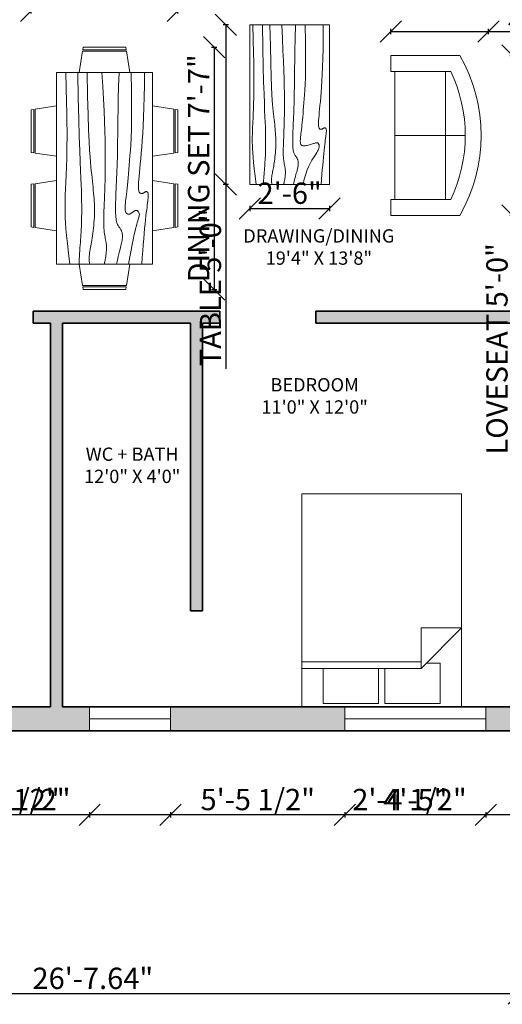
# Model space of a CAD drawing. Units: inches. Extents: x 2561 to 3163, y 493 to 1211.
# Tile 2 of 8: x 2762 to 2943, y 512 to 882. Entities that reach past the tile are written whole.
import ezdxf

# ---------------------------------------------------------------- set-up
doc = ezdxf.new("R2010")
doc.units = ezdxf.units.IN
for name, color, linetype, lineweight in [('A-ANNO-DIMS', 2, 'Continuous', 18), ('A-AREA-IDEN', 7, 'Continuous', 18), ('A-FURN', 8, 'Continuous', 18), ('A-GLAZ', 4, 'Continuous', 18), ('A-WALL', 7, 'Continuous', 35), ('A-WALL-PATT', 24, 'Continuous', 13)]:
    doc.layers.add(name, color=color, linetype=linetype, lineweight=lineweight)
doc.styles.get("Standard").update_dxf_attribs({"font": 'arial.ttf'})
doc.dimstyles.new('ISO-25', dxfattribs={"dimtxt": 8, "dimasz": 8, "dimexe": 1, "dimexo": 1, "dimtad": 1, "dimlunit": 3, "dimtxsty": 'Standard', "dimblk": 'OBLIQUE', "dimcen": 2.5, "dimadec": 0, "dimazin": 0, "dimtfac": 1, "dimtmove": 0, "dimatfit": 3, "dimfxl": 1, "dimfxlon": 1, "dimarcsym": 0})

# ---------------------------------------------------------------- blocks, each defined once
blk = doc.blocks.new('Table - Rectangular Woodgrain 60 x 30 in.')
for p, q in [((0, 0), (0, -30)), ((60, 0), (0, 0)), ((60, -30), (60, 0)), ((0, -30), (60, -30))]:
    blk.add_line(p, q)
for points in [[(0, -2.4), (4.8155, -2.418), (9.0302, -2.4688), (12.709, -2.5477), (15.9167, -2.65), (18.7181, -2.7711), (21.1781, -2.9063), (23.3616, -3.0508), (25.3333, -3.2), (27.1477, -3.3495), (28.8172, -3.4958), (30.3437, -3.636), (31.7291, -3.7667), (32.9756, -3.8849), (34.0849, -3.9875), (35.059, -4.0714), (35.9, -4.1334), (36.6114, -4.1711), (37.2041, -4.1854), (37.6906, -4.1779), (38.0833, -4.15), (38.3948, -4.1034), (38.6375, -4.0396), (38.8239, -3.9602), (38.9666, -3.8667), (39.0764, -3.7608), (39.1573, -3.6448), (39.2116, -3.521), (39.2416, -3.3917), (39.2498, -3.2593), (39.2385, -3.1261), (39.21, -2.9944), (39.1666, -2.8667), (39.111, -2.7447), (39.0468, -2.6281), (38.978, -2.5163), (38.9083, -2.4083), (38.8418, -2.3035), (38.7823, -2.201), (38.7337, -2.1001), (38.7, -2), (38.6844, -1.9003), (38.6875, -1.8021), (38.7094, -1.707), (38.75, -1.6167), (38.8094, -1.5326), (38.8875, -1.4563), (38.9844, -1.3893), (39.1, -1.3333), (39.2351, -1.2896), (39.3937, -1.2583), (39.5804, -1.2396), (39.8, -1.2333), (40.057, -1.2396), (40.3562, -1.2583), (40.7023, -1.2896), (41.1, -1.3333), (41.5547, -1.3895), (42.0755, -1.4573), (42.6721, -1.5361), (43.3542, -1.625), (44.1316, -1.7233), (45.014, -1.8302), (46.0114, -1.9449), (47.1333, -2.0667), (48.3862, -2.1947), (49.7625, -2.3281), (51.2513, -2.4663), (52.8416, -2.6083), (54.5226, -2.7535), (56.2833, -2.9011), (58.1127, -3.0501), (60, -3.2)], [(0, -9.2), (6.5759, -9.0858), (11.9385, -9.0365), (16.2527, -9.0418), (19.6833, -9.0917), (22.3952, -9.1759), (24.5531, -9.2844), (26.322, -9.4069), (27.8666, -9.5333), (29.3241, -9.6553), (30.7203, -9.7719), (32.0532, -9.8837), (33.3208, -9.9917), (34.5213, -10.0965), (35.6526, -10.199), (36.7128, -10.2999), (37.7, -10.4), (38.6129, -10.4996), (39.4531, -10.5969), (40.223, -10.6895), (40.925, -10.775), (41.5613, -10.8512), (42.1344, -10.9156), (42.6465, -10.966), (43.1, -11), (43.4976, -11.0158), (43.8437, -11.0136), (44.143, -10.9942), (44.4, -10.9583), (44.6195, -10.9069), (44.8062, -10.8406), (44.9648, -10.7603), (45.1, -10.6667), (45.2155, -10.5598), (45.3114, -10.4365), (45.3871, -10.2929), (45.4416, -10.125), (45.4743, -9.929), (45.4844, -9.7011), (45.4709, -9.4371), (45.4333, -9.1333), (45.3716, -8.7883), (45.2896, -8.4104), (45.1919, -8.0107), (45.0833, -7.6), (44.9685, -7.1893), (44.8521, -6.7896), (44.7388, -6.4117), (44.6333, -6.0667), (44.54, -5.7628), (44.4614, -5.4979), (44.4001, -5.2675), (44.3583, -5.0667), (44.3384, -4.8909), (44.3427, -4.7354), (44.3736, -4.5956), (44.4333, -4.4667), (44.5236, -4.3453), (44.6427, -4.2333), (44.7884, -4.1339), (44.9583, -4.05), (45.1501, -3.9849), (45.3614, -3.9417), (45.59, -3.9234), (45.8333, -3.9333), (46.0915, -3.9749), (46.3734, -4.0531), (46.6906, -4.1736), (47.0542, -4.3417), (47.4756, -4.5629), (47.9661, -4.8427), (48.5372, -5.1866), (49.2, -5.6), (49.9676, -6.0844), (50.8594, -6.625), (51.8965, -7.2031), (53.1, -7.8), (54.491, -8.3969), (56.0906, -8.975), (57.9199, -9.5156), (60, -10)], [(0, -12.8), (5.1847, -12.9322), (9.6213, -13.0323), (13.3963, -13.1059), (16.5958, -13.1583), (19.3063, -13.1952), (21.614, -13.2219), (23.6054, -13.2439), (25.3666, -13.2667), (26.9728, -13.2947), (28.4531, -13.3281), (29.8256, -13.3663), (31.1083, -13.4083), (32.3191, -13.4535), (33.476, -13.501), (34.597, -13.5501), (35.7, -13.6), (36.7984, -13.6497), (37.8875, -13.6979), (38.9578, -13.743), (40, -13.7833), (41.0047, -13.8174), (41.9625, -13.8438), (42.864, -13.8607), (43.7, -13.8667), (44.4631, -13.8604), (45.1552, -13.8417), (45.7801, -13.8104), (46.3416, -13.7667), (46.8439, -13.7104), (47.2906, -13.6417), (47.6858, -13.5604), (48.0333, -13.4667), (48.3375, -13.3608), (48.6042, -13.2448), (48.8396, -13.121), (49.05, -12.9917), (49.2417, -12.8593), (49.4208, -12.7261), (49.5937, -12.5944), (49.7667, -12.4667), (49.9452, -12.3451), (50.1323, -12.2313), (50.3303, -12.1268), (50.5416, -12.0333), (50.7686, -11.9524), (51.0135, -11.8854), (51.2788, -11.8341), (51.5666, -11.8), (51.8785, -11.7843), (52.2116, -11.7865), (52.562, -11.8059), (52.926, -11.8417), (53.2998, -11.8931), (53.6795, -11.9594), (54.0614, -12.0397), (54.4416, -12.1333), (54.8223, -12.2401), (55.2293, -12.3625), (55.6942, -12.5037), (56.2489, -12.6667), (56.9251, -12.8547), (57.7545, -13.0708), (58.7689, -13.3182), (60, -13.6)], [(0, -18), (5.124, -17.7273), (9.6609, -17.5057), (13.6705, -17.3303), (17.2125, -17.1958), (20.3467, -17.0973), (23.1328, -17.0297), (25.6307, -16.9878), (27.9, -16.9667), (29.9928, -16.9617), (31.9302, -16.9703), (33.7254, -16.9907), (35.3917, -17.0208), (36.9423, -17.0588), (38.3906, -17.1026), (39.7499, -17.1503), (41.0333, -17.2), (42.2519, -17.2496), (43.4073, -17.2969), (44.4986, -17.3395), (45.525, -17.375), (46.4858, -17.4012), (47.3802, -17.4156), (48.2074, -17.416), (48.9667, -17.4), (49.6583, -17.3662), (50.2872, -17.3167), (50.8595, -17.2547), (51.3812, -17.1833), (51.8584, -17.1057), (52.2971, -17.025), (52.7034, -16.9443), (53.0833, -16.8667), (53.443, -16.7951), (53.789, -16.7313), (54.128, -16.6768), (54.4666, -16.6334), (54.8115, -16.6024), (55.1693, -16.5854), (55.5465, -16.5841), (55.95, -16.6), (56.3828, -16.6337), (56.8346, -16.6823), (57.2915, -16.7418), (57.7396, -16.8084), (58.165, -16.878), (58.5539, -16.9469), (58.8924, -17.0111), (59.1666, -17.0667), (59.3679, -17.1107), (59.5078, -17.1438), (59.6032, -17.1675), (59.6708, -17.1833), (59.7275, -17.193), (59.7901, -17.1979), (59.8753, -17.1998), (60, -17.2)], [(0, -22.4), (8.0098, -22.2501), (14.4094, -22.1011), (19.4168, -21.9535), (23.25, -21.8083), (26.1269, -21.6663), (28.2656, -21.5281), (29.884, -21.3947), (31.2, -21.2667), (32.3967, -21.1448), (33.5172, -21.0292), (34.5697, -20.9198), (35.5625, -20.8167), (36.5037, -20.7198), (37.4015, -20.6292), (38.2642, -20.5448), (39.1, -20.4667), (39.9164, -20.3951), (40.7187, -20.3313), (41.5117, -20.2768), (42.3, -20.2333), (43.0883, -20.2024), (43.8812, -20.1854), (44.6836, -20.1841), (45.5, -20.2), (46.3328, -20.234), (47.1747, -20.2844), (48.0163, -20.3488), (48.8479, -20.425), (49.66, -20.5106), (50.4429, -20.6031), (51.1872, -20.7004), (51.8833, -20.8), (52.5246, -20.8999), (53.1166, -20.9995), (53.6681, -21.0983), (54.1875, -21.1958), (54.6834, -21.2919), (55.1646, -21.3859), (55.6394, -21.4777), (56.1167, -21.5667), (56.6028, -21.6515), (57.0961, -21.7266), (57.5929, -21.7852), (58.0896, -21.8208), (58.5823, -21.8268), (59.0674, -21.7964), (59.5412, -21.723), (60, -21.6)], [(0, -25.2), (8.6355, -25.0504), (15.7026, -24.9031), (21.4049, -24.7606), (25.9458, -24.625), (29.529, -24.4988), (32.3578, -24.3844), (34.6359, -24.284), (36.5667, -24.2), (38.3213, -24.1341), (39.9417, -24.0854), (41.437, -24.0523), (42.8167, -24.0333), (44.0901, -24.0268), (45.2667, -24.0313), (46.3557, -24.0451), (47.3667, -24.0667), (48.309, -24.0947), (49.1928, -24.1287), (50.0284, -24.168), (50.826, -24.2125), (51.5959, -24.2617), (52.3483, -24.3151), (53.0935, -24.3725), (53.8417, -24.4334), (54.6009, -24.497), (55.3699, -24.561), (56.1454, -24.6226), (56.9239, -24.6792), (57.7021, -24.7279), (58.4764, -24.7662), (59.2435, -24.7911), (60, -24.8)], [(0, -28.8), (5.6867, -28.6681), (10.45, -28.5698), (14.407, -28.5012), (17.675, -28.4584), (20.3711, -28.4374), (22.6125, -28.4344), (24.5164, -28.4455), (26.2, -28.4667), (27.762, -28.4947), (29.2276, -28.5281), (30.6033, -28.5663), (31.8958, -28.6084), (33.1118, -28.6535), (34.2578, -28.7011), (35.3405, -28.7501), (36.3666, -28.8), (37.3443, -28.8497), (38.288, -28.8974), (39.2137, -28.9412), (40.1375, -28.9792), (41.0753, -29.0093), (42.0432, -29.0297), (43.0572, -29.0384), (44.1333, -29.0333), (45.2936, -29.0114), (46.5843, -28.9641), (48.0579, -28.8816), (49.7666, -28.7542), (51.7629, -28.5721), (54.0989, -28.3255), (56.8272, -28.0048), (60, -27.6)]]:
    blk.add_lwpolyline(points)
blk = doc.blocks.new('Sofa - Roundback Loveseat 5 ft.')
for p, q in [((0, -32.44198), (0, -5.99998)), ((-24, -33.99998), (-24, -11.46958)), ((-23.9998, -13.38178), (23.99986, -13.38178)), ((24.00004, -33.99998), (24.00004, -11.46958)), ((-24, -32.44198), (24.00004, -32.44198))]:
    blk.add_line(p, q)
for points in [[(-24, -33.99998), (-30, -33.99998), (-30, -7.99998)], [(30.00004, -7.99998), (30.00004, -33.99998), (24.00004, -33.99998)]]:
    blk.add_lwpolyline(points)
for centre, radius, start, end in [((0, -60.24998), 60.24998, 60.13715, 119.8628), ((0, -61.38438), 55.38444, 64.32083, 115.6792)]:
    blk.add_arc(centre, radius, start, end)
blk = doc.blocks.new('Dining Set - 36 x 72 in.')
for p, q in [((-22.2343, 26.00059), (-23.4847, 17.99762)), ((-22.2304, 26), (-5.7608, 26)), ((-22, 27.5), (-22.1562, 26.50042)), ((-5.8416, 26.5), (-22.1534, 26.5)), ((-22, 27.5), (-6, 27.5)), ((-5.8437, 26.49966), (-6, 27.5)), ((-4.5152, 17.99762), (-5.7655, 25.99926)), ((5.7657, 26.00059), (4.5153, 17.99762)), ((5.7696, 26), (22.2392, 26)), ((6, 27.5), (5.8438, 26.50042)), ((22.1584, 26.5), (5.8466, 26.5)), ((6, 27.5), (22, 27.5)), ((22.1563, 26.49966), (22, 27.5)), ((23.4848, 17.99762), (22.2345, 25.99926)), ((36, 18), (-36, 18)), ((-36, 18), (-36, -18)), ((36, -18), (36, 18)), ((-45.5, 8), (-44.5004, 8.15617)), ((-45.5, 8), (-45.5, -8)), ((-44.5, -8.15843), (-44.5, 8.15338)), ((-44.0006, 8.23428), (-35.9976, 9.48474)), ((-44, 8.23041), (-44, -8.23915)), ((44.0006, 8.23428), (35.9976, 9.48474)), ((44, 8.23041), (44, -8.23915)), ((44.5, -8.15843), (44.5, 8.15338)), ((45.5, 8), (44.5005, 8.15617)), ((45.5, 8), (45.5, -8)), ((-44.4997, -8.15631), (-45.5, -8)), ((-35.9976, -9.48476), (-43.9993, -8.2345)), ((35.9976, -9.48476), (43.9993, -8.2345)), ((44.4997, -8.15631), (45.5, -8)), ((-36, -18), (36, -18)), ((-22.2343, -26.0006), (-23.4847, -17.99762)), ((-4.5152, -17.99762), (-5.7655, -25.99928)), ((5.7657, -26.0006), (4.5153, -17.99762)), ((23.4848, -17.99762), (22.2345, -25.99928)), ((-22.2304, -26), (-5.7608, -26)), ((-22, -27.5), (-22.1562, -26.50044)), ((-5.8416, -26.5), (-22.1534, -26.5)), ((-22, -27.5), (-6, -27.5)), ((-5.8437, -26.49967), (-6, -27.5)), ((5.7696, -26), (22.2392, -26)), ((6, -27.5), (5.8438, -26.50044)), ((22.1584, -26.5), (5.8466, -26.5)), ((6, -27.5), (22, -27.5)), ((22.1563, -26.49967), (22, -27.5))]:
    blk.add_line(p, q)
for points in [[(-36, 15), (-31.1772, 14.97754), (-26.8079, 14.91406), (-22.8538, 14.81543), (-19.276, 14.6875), (-16.0362, 14.53613), (-13.0957, 14.36718), (-10.4159, 14.18652), (-7.9583, 14), (-5.6904, 13.81315), (-3.6035, 13.63021), (-1.6954, 13.45508), (0.0365, 13.29166), (1.5945, 13.14388), (2.9811, 13.01562), (4.1988, 12.9108), (5.25, 12.83333), (6.1393, 12.78613), (6.8802, 12.76823), (7.4883, 12.77767), (7.9792, 12.8125), (8.3685, 12.87077), (8.6719, 12.95052), (8.9049, 13.0498), (9.0833, 13.16666), (9.2205, 13.29899), (9.3216, 13.44401), (9.3895, 13.59879), (9.4271, 13.76041), (9.4373, 13.92594), (9.4232, 14.09245), (9.3875, 14.257), (9.3333, 14.41666), (9.2638, 14.56917), (9.1836, 14.71484), (9.0975, 14.85465), (9.0104, 14.98958), (8.9272, 15.1206), (8.8529, 15.2487), (8.7922, 15.37483), (8.75, 15.5), (8.7305, 15.62467), (8.7344, 15.74739), (8.7617, 15.86621), (8.8125, 15.97916), (8.8867, 16.08431), (8.9844, 16.17968), (9.1055, 16.26334), (9.25, 16.33333), (9.4189, 16.38802), (9.6172, 16.42708), (9.8506, 16.45052), (10.125, 16.45833), (10.4463, 16.45052), (10.8203, 16.42708), (11.2529, 16.38802), (11.75, 16.33333), (12.3184, 16.26318), (12.9694, 16.17838), (13.7151, 16.07991), (14.5677, 15.96875), (15.5395, 15.84586), (16.6426, 15.71224), (17.8893, 15.56884), (19.2917, 15.41666), (20.859, 15.25667), (22.5879, 15.08984), (24.4721, 14.91715), (26.5052, 14.73958), (28.6809, 14.5581), (30.9929, 14.3737), (33.4347, 14.18733), (36, 14)], [(-36, 10), (-28.9766, 10.14274), (-23.1725, 10.20442), (-18.4241, 10.19775), (-14.5677, 10.13541), (-11.4399, 10.03011), (-8.877, 9.89453), (-6.7154, 9.74137), (-4.7917, 9.58333), (-2.9698, 9.43082), (-1.2246, 9.28515), (0.4415, 9.14534), (2.026, 9.01041), (3.5266, 8.87939), (4.9408, 8.7513), (6.266, 8.62516), (7.5, 8.5), (8.6411, 8.37549), (9.6914, 8.2539), (10.6538, 8.13818), (11.5312, 8.03125), (12.3267, 7.93603), (13.043, 7.85547), (13.6831, 7.79248), (14.25, 7.75), (14.7471, 7.7303), (15.1797, 7.73307), (15.5537, 7.75732), (15.875, 7.80208), (16.1494, 7.86637), (16.3828, 7.94922), (16.5811, 8.04964), (16.75, 8.16666), (16.8944, 8.29915), (17.0143, 8.44531), (17.1089, 8.60319), (17.1771, 8.77083), (17.218, 8.94629), (17.2305, 9.1276), (17.2137, 9.31282), (17.1667, 9.5), (17.0895, 9.6875), (16.987, 9.875), (16.8649, 10.0625), (16.7292, 10.25), (16.5856, 10.4375), (16.4401, 10.625), (16.2985, 10.8125), (16.1667, 11), (16.05, 11.18733), (15.9518, 11.3737), (15.8752, 11.5581), (15.8229, 11.73958), (15.798, 11.91715), (15.8034, 12.08984), (15.842, 12.25667), (15.9167, 12.41666), (16.0295, 12.56836), (16.1784, 12.70833), (16.3605, 12.83268), (16.5729, 12.9375), (16.8127, 13.01888), (17.0768, 13.07291), (17.3625, 13.0957), (17.6667, 13.08333), (17.9894, 13.03312), (18.3418, 12.94726), (18.7382, 12.82918), (19.1927, 12.68229), (19.7195, 12.51001), (20.3327, 12.31575), (21.0465, 12.10294), (21.875, 11.875), (22.8357, 11.63354), (23.959, 11.37304), (25.2786, 11.08618), (26.8282, 10.76562), (28.6414, 10.40405), (30.752, 9.99414), (33.1936, 9.52856), (36, 9)], [(-36, 5.5), (-30.7157, 5.3348), (-26.069, 5.20963), (-21.9946, 5.11767), (-18.4271, 5.05208), (-15.3009, 5.00602), (-12.5508, 4.97265), (-10.1112, 4.94515), (-7.9167, 4.91666), (-5.909, 4.88167), (-4.0586, 4.83984), (-2.3429, 4.79215), (-0.7396, 4.73958), (0.7739, 4.6831), (2.22, 4.6237), (3.6213, 4.56233), (5, 4.5), (6.373, 4.43782), (7.7344, 4.3776), (9.0723, 4.32129), (10.375, 4.27083), (11.6309, 4.22819), (12.8281, 4.19531), (13.9551, 4.17415), (15, 4.16666), (15.954, 4.17448), (16.819, 4.19791), (17.6001, 4.23698), (18.3021, 4.29166), (18.9299, 4.36198), (19.4883, 4.44791), (19.9823, 4.54948), (20.4167, 4.66666), (20.7969, 4.79899), (21.1302, 4.94401), (21.4245, 5.09879), (21.6875, 5.26041), (21.9271, 5.42594), (22.1511, 5.59245), (22.3672, 5.757), (22.5834, 5.91666), (22.8065, 6.06868), (23.0404, 6.21093), (23.2879, 6.34147), (23.5521, 6.45833), (23.8358, 6.55957), (24.142, 6.64323), (24.4735, 6.70735), (24.8334, 6.75), (25.2235, 6.76969), (25.642, 6.76692), (26.0858, 6.74267), (26.5521, 6.69791), (27.0379, 6.63362), (27.5404, 6.55078), (28.0565, 6.45036), (28.5834, 6.33333), (29.1242, 6.19987), (29.7071, 6.04687), (30.3661, 5.87044), (31.1354, 5.66666), (32.0493, 5.43164), (33.142, 5.16146), (34.4475, 4.85221), (36, 4.5)], [(-36, -1), (-30.7915, -0.6591), (-26.0195, -0.38216), (-21.6519, -0.16284), (-17.6563, 0.00521), (-14.0005, 0.12833), (-10.6523, 0.21289), (-7.5796, 0.26522), (-4.75, 0.29166), (-2.134, 0.29793), (0.2878, 0.28711), (2.5317, 0.26163), (4.6146, 0.22396), (6.5529, 0.17651), (8.3633, 0.12174), (10.0623, 0.06209), (11.6667, 0), (13.1899, -0.06201), (14.6341, -0.1211), (15.9982, -0.17432), (17.2813, -0.21875), (18.4823, -0.25147), (19.6003, -0.26953), (20.6343, -0.27002), (21.5834, -0.25), (22.4481, -0.20768), (23.2357, -0.14584), (23.9549, -0.06836), (24.6146, 0.02083), (25.2235, 0.11784), (25.7904, 0.21875), (26.3241, 0.31966), (26.8334, 0.41666), (27.3265, 0.50618), (27.8099, 0.58593), (28.2894, 0.65397), (28.7709, 0.70833), (29.2601, 0.74707), (29.763, 0.76823), (30.2855, 0.76985), (30.8334, 0.75), (31.4088, 0.70784), (31.9994, 0.64713), (32.589, 0.57275), (33.1615, 0.48958), (33.7008, 0.4025), (34.1908, 0.3164), (34.6153, 0.23616), (34.9584, 0.16666), (35.2099, 0.11165), (35.3848, 0.07031), (35.504, 0.04069), (35.5886, 0.02083), (35.6594, 0.00879), (35.7377, 0.0026), (35.8442, 0.00032), (36, 0)], [(-36, -6.5), (-27.1843, -6.31267), (-20.084, -6.1263), (-14.469, -5.9419), (-10.1094, -5.76042), (-6.7752, -5.58285), (-4.2363, -5.41016), (-2.2629, -5.24333), (-0.625, -5.08334), (0.8708, -4.93099), (2.2715, -4.78646), (3.5872, -4.64974), (4.8281, -4.52084), (6.0046, -4.39974), (7.127, -4.28646), (8.2053, -4.18099), (9.25, -4.08334), (10.2705, -3.99382), (11.2734, -3.91407), (12.2647, -3.84603), (13.25, -3.79167), (14.2354, -3.75293), (15.2266, -3.73177), (16.2295, -3.73015), (17.25, -3.75), (18.2912, -3.79248), (19.3451, -3.85547), (20.4009, -3.93604), (21.4479, -4.03125), (22.4754, -4.13819), (23.4727, -4.25391), (24.4289, -4.37549), (25.3334, -4.5), (26.1785, -4.62492), (26.9694, -4.74935), (27.7145, -4.87281), (28.4219, -4.99479), (29.1, -5.11483), (29.7572, -5.23242), (30.4016, -5.34709), (31.0417, -5.45834), (31.6837, -5.56437), (32.3262, -5.65821), (32.9658, -5.73153), (33.599, -5.77604), (34.2224, -5.78345), (34.8327, -5.74545), (35.4264, -5.65373), (36, -5.5)], [(-36, -10), (-26.4022, -9.81299), (-18.4675, -9.62891), (-11.9839, -9.45069), (-6.7396, -9.28125), (-2.5226, -9.12354), (0.8789, -8.98047), (3.6769, -8.85498), (6.0833, -8.75), (8.2767, -8.66765), (10.3021, -8.60677), (12.1712, -8.56543), (13.8958, -8.54167), (15.4876, -8.53353), (16.9583, -8.53907), (18.3197, -8.55632), (19.5834, -8.58334), (20.7616, -8.61841), (21.8685, -8.66081), (22.9188, -8.71004), (23.9271, -8.76563), (24.9081, -8.82707), (25.8763, -8.89388), (26.8465, -8.96558), (27.8334, -9.04167), (28.8474, -9.12118), (29.8828, -9.20117), (30.93, -9.27824), (31.9792, -9.34896), (33.0205, -9.40991), (34.0443, -9.45768), (35.0407, -9.48885), (36, -9.5)], [(-36, -14.5), (-30.0881, -14.33513), (-25.0332, -14.21224), (-20.7312, -14.12647), (-17.0781, -14.07292), (-13.97, -14.04671), (-11.3027, -14.04297), (-8.9724, -14.05681), (-6.875, -14.08334), (-4.9224, -14.11833), (-3.0905, -14.16016), (-1.3709, -14.20785), (0.2448, -14.26042), (1.7647, -14.3169), (3.1973, -14.3763), (4.5507, -14.43767), (5.8333, -14.5), (7.0554, -14.5621), (8.235, -14.62175), (9.3922, -14.67652), (10.5469, -14.72396), (11.7192, -14.76164), (12.929, -14.78711), (14.1965, -14.79794), (15.5417, -14.79167), (16.9933, -14.76424), (18.6152, -14.70508), (20.4804, -14.60197), (22.6615, -14.44271), (25.2312, -14.21509), (28.2624, -13.9069), (31.8277, -13.50594), (36, -13)]]:
    blk.add_lwpolyline(points)
blk = doc.blocks.new('Bed - Queen')
for p, q in [((0, -80.00003), (0, 0)), ((0, 0), (59.99999, 0)), ((59.99999, 0), (59.99999, -80.00003)), ((7.99999, -1.2), (28.79998, -1.2)), ((7.99999, -14.4), (7.99999, -1.2)), ((28.79998, -1.2), (28.79998, -14.4)), ((31.19999, -1.2), (51.99999, -1.2)), ((31.19999, -14.4), (31.19999, -1.2)), ((51.99999, -1.2), (51.99999, -16.4)), ((0, -14.4), (44.8, -14.4)), ((59.99999, -29.6), (44.8, -14.4)), ((44.8, -14.4), (44.8, -29.6)), ((44.8, -16.8), (0, -16.8)), ((51.99999, -16.4), (46.79936, -16.4)), ((44.8, -29.6), (59.99999, -29.6)), ((59.99999, -80.00003), (0, -80.00003))]:
    blk.add_line(p, q)
blk = doc.blocks.new('_Oblique')
at = {"color": 0, "linetype": 'ByBlock', "lineweight": -2}
blk.add_line((-0.5, -0.5), (0.5, 0.5), dxfattribs=at)
blk = doc.blocks.new('*D15')
at = {"layer": 'A-ANNO-DIMS', "color": 0, "lineweight": -2, "transparency": 16777216}
for p, q in [((2629.27, 516.82), (2629.27, 514.82)), ((2629.27, 515.82), (2948.92, 515.82)), ((2948.92, 516.82), (2948.92, 514.82))]:
    blk.add_line(p, q, dxfattribs=at)
at = {"layer": 'Defpoints', "color": 0, "transparency": 16777216}
for p in [(2629.27, 614.57), (2948.92, 614.57), (2948.92, 515.82)]:
    blk.add_point(p, dxfattribs=at)
at = {"layer": 'A-ANNO-DIMS', "color": 0, "lineweight": -2, "transparency": 16777216, "xscale": 8, "yscale": 8, "zscale": 8, "rotation": 180}
blk.add_blockref('_Oblique', (2629.27, 515.82), dxfattribs=at)
at = {"layer": 'A-ANNO-DIMS', "color": 0, "lineweight": -2, "transparency": 16777216, "xscale": 8, "yscale": 8, "zscale": 8}
blk.add_blockref('_Oblique', (2948.92, 515.82), dxfattribs=at)
at = {"layer": 'A-ANNO-DIMS', "color": 0, "transparency": 16777216, "insert": (2789.1, 520.53), "char_height": 8, "attachment_point": 5}
blk.add_mtext('26\'-7.64"', dxfattribs=at)
blk = doc.blocks.new('*D17')
at = {"layer": 'A-ANNO-DIMS', "color": 0, "lineweight": -2, "transparency": 16777216}
for p, q in [((2571.63, 1093.07), (2569.63, 1093.07)), ((2570.63, 1093.07), (2570.63, 529.07)), ((2571.63, 529.07), (2569.63, 529.07))]:
    blk.add_line(p, q, dxfattribs=at)
at = {"layer": 'Defpoints', "color": 0, "transparency": 16777216}
for p in [(2629.27, 1093.07), (2570.63, 529.07), (3109.27, 529.07)]:
    blk.add_point(p, dxfattribs=at)
at = {"layer": 'A-ANNO-DIMS', "color": 0, "lineweight": -2, "transparency": 16777216, "xscale": 8, "yscale": 8, "zscale": 8}
for p, rotation in [((2570.63, 1093.07), 90), ((2570.63, 529.07), 270)]:
    blk.add_blockref('_Oblique', p, dxfattribs=dict(at, rotation=rotation))
at = {"layer": 'A-ANNO-DIMS', "color": 0, "transparency": 16777216, "insert": (2566, 811.07), "char_height": 8, "attachment_point": 5, "rotation": 90}
blk.add_mtext("47'", dxfattribs=at)
blk = doc.blocks.new('*D24')
at = {"layer": 'A-ANNO-DIMS', "color": 0, "lineweight": -2, "transparency": 16777216}
for p, q in [((2839.96, 879.66), (2837.96, 879.66)), ((2838.96, 879.66), (2838.96, 819.66)), ((2839.96, 819.66), (2837.96, 819.66)), ((2838.96, 819.66), (2838.96, 750.44))]:
    blk.add_line(p, q, dxfattribs=at)
at = {"layer": 'Defpoints', "color": 0, "transparency": 16777216}
for p in [(2847.96, 879.66), (2838.96, 819.66), (2847.96, 819.66)]:
    blk.add_point(p, dxfattribs=at)
at = {"layer": 'A-ANNO-DIMS', "color": 0, "lineweight": -2, "transparency": 16777216, "xscale": 8, "yscale": 8, "zscale": 8}
for p, rotation in [((2838.96, 879.66), 90), ((2838.96, 819.66), 270)]:
    blk.add_blockref('_Oblique', p, dxfattribs=dict(at, rotation=rotation))
at = {"layer": 'A-ANNO-DIMS', "color": 0, "transparency": 16777216, "insert": (2834.25, 781.05), "char_height": 8, "attachment_point": 5, "rotation": 90}
blk.add_mtext('TABLE 5\'-0"', dxfattribs=at)
blk = doc.blocks.new('*D25')
at = {"layer": 'A-ANNO-DIMS', "color": 0, "lineweight": -2, "transparency": 16777216}
for p, q in [((2847.96, 811.66), (2847.96, 809.66)), ((2847.96, 810.66), (2877.96, 810.66)), ((2877.96, 811.66), (2877.96, 809.66))]:
    blk.add_line(p, q, dxfattribs=at)
at = {"layer": 'Defpoints', "color": 0, "transparency": 16777216}
for p in [(2847.96, 819.66), (2877.96, 819.66), (2877.96, 810.66)]:
    blk.add_point(p, dxfattribs=at)
at = {"layer": 'A-ANNO-DIMS', "color": 0, "lineweight": -2, "transparency": 16777216, "xscale": 8, "yscale": 8, "zscale": 8, "rotation": 180}
blk.add_blockref('_Oblique', (2847.96, 810.66), dxfattribs=at)
at = {"layer": 'A-ANNO-DIMS', "color": 0, "lineweight": -2, "transparency": 16777216, "xscale": 8, "yscale": 8, "zscale": 8}
blk.add_blockref('_Oblique', (2877.96, 810.66), dxfattribs=at)
at = {"layer": 'A-ANNO-DIMS', "color": 0, "transparency": 16777216, "insert": (2862.96, 815.37), "char_height": 8, "attachment_point": 5}
blk.add_mtext('2\'-6"', dxfattribs=at)
blk = doc.blocks.new('*D26')
at = {"layer": 'A-ANNO-DIMS', "color": 0, "lineweight": -2, "transparency": 16777216}
for p, q in [((2945.53, 868.1), (2947.53, 868.1)), ((2946.53, 868.1), (2946.53, 808.1)), ((2945.53, 808.1), (2947.53, 808.1)), ((2946.53, 808.1), (2946.53, 715.83))]:
    blk.add_line(p, q, dxfattribs=at)
at = {"layer": 'Defpoints', "color": 0, "transparency": 16777216}
for p in [(2937.53, 868.1), (2937.53, 808.1), (2946.53, 808.1)]:
    blk.add_point(p, dxfattribs=at)
at = {"layer": 'A-ANNO-DIMS', "color": 0, "lineweight": -2, "transparency": 16777216, "xscale": 8, "yscale": 8, "zscale": 8}
for p, rotation in [((2946.53, 868.1), 90), ((2946.53, 808.1), 270)]:
    blk.add_blockref('_Oblique', p, dxfattribs=dict(at, rotation=rotation))
at = {"layer": 'A-ANNO-DIMS', "color": 0, "transparency": 16777216, "insert": (2941.77, 757.96), "char_height": 8, "attachment_point": 5, "rotation": 90}
blk.add_mtext('LOVESEAT 5\'-0"', dxfattribs=at)
blk = doc.blocks.new('*D27')
at = {"layer": 'A-ANNO-DIMS', "color": 0, "lineweight": -2, "transparency": 16777216}
for p, q in [((2900.86, 876.1), (2900.86, 878.1)), ((2900.86, 877.1), (2937.53, 877.1)), ((2937.53, 876.1), (2937.53, 878.1)), ((2937.53, 877.1), (2986.68, 877.1))]:
    blk.add_line(p, q, dxfattribs=at)
at = {"layer": 'Defpoints', "color": 0, "transparency": 16777216}
for p in [(2937.53, 877.1), (2900.86, 868.1), (2937.53, 868.1)]:
    blk.add_point(p, dxfattribs=at)
at = {"layer": 'A-ANNO-DIMS', "color": 0, "lineweight": -2, "transparency": 16777216, "xscale": 8, "yscale": 8, "zscale": 8, "rotation": 180}
blk.add_blockref('_Oblique', (2900.86, 877.1), dxfattribs=at)
at = {"layer": 'A-ANNO-DIMS', "color": 0, "lineweight": -2, "transparency": 16777216, "xscale": 8, "yscale": 8, "zscale": 8}
blk.add_blockref('_Oblique', (2937.53, 877.1), dxfattribs=at)
at = {"layer": 'A-ANNO-DIMS', "color": 0, "transparency": 16777216, "insert": (2966.11, 881.86), "char_height": 8, "attachment_point": 5}
blk.add_mtext('3\'-0 1/2"', dxfattribs=at)
blk = doc.blocks.new('*D28')
at = {"layer": 'A-ANNO-DIMS', "color": 0, "lineweight": -2, "transparency": 16777216}
for p, q in [((2833.61, 871.24), (2835.61, 871.24)), ((2834.61, 871.24), (2834.61, 780.24)), ((2833.61, 780.24), (2835.61, 780.24))]:
    blk.add_line(p, q, dxfattribs=at)
at = {"layer": 'Defpoints', "color": 0, "transparency": 16777216}
for p in [(2820.96, 871.24), (2820.96, 780.24), (2834.61, 780.24)]:
    blk.add_point(p, dxfattribs=at)
at = {"layer": 'A-ANNO-DIMS', "color": 0, "lineweight": -2, "transparency": 16777216, "xscale": 8, "yscale": 8, "zscale": 8}
for p, rotation in [((2834.61, 871.24), 90), ((2834.61, 780.24), 270)]:
    blk.add_blockref('_Oblique', p, dxfattribs=dict(at, rotation=rotation))
at = {"layer": 'A-ANNO-DIMS', "color": 0, "transparency": 16777216, "insert": (2829.85, 825.74), "char_height": 8, "attachment_point": 5, "rotation": 90}
blk.add_mtext('DINING SET 7\'-7"', dxfattribs=at)
blk = doc.blocks.new('*D29')
at = {"layer": 'A-ANNO-DIMS', "color": 0, "lineweight": -2, "transparency": 16777216}
for p, q in [((2765.96, 883.89), (2765.96, 885.89)), ((2765.96, 884.89), (2820.96, 884.89)), ((2820.96, 883.89), (2820.96, 885.89))]:
    blk.add_line(p, q, dxfattribs=at)
at = {"layer": 'Defpoints', "color": 0, "transparency": 16777216}
for p in [(2820.96, 884.89), (2765.96, 871.24), (2820.96, 871.24)]:
    blk.add_point(p, dxfattribs=at)
at = {"layer": 'A-ANNO-DIMS', "color": 0, "lineweight": -2, "transparency": 16777216, "xscale": 8, "yscale": 8, "zscale": 8, "rotation": 180}
blk.add_blockref('_Oblique', (2765.96, 884.89), dxfattribs=at)
at = {"layer": 'A-ANNO-DIMS', "color": 0, "lineweight": -2, "transparency": 16777216, "xscale": 8, "yscale": 8, "zscale": 8}
blk.add_blockref('_Oblique', (2820.96, 884.89), dxfattribs=at)
at = {"layer": 'A-ANNO-DIMS', "color": 0, "transparency": 16777216, "insert": (2793.46, 889.52), "char_height": 8, "attachment_point": 5}
blk.add_mtext('4\'-7"', dxfattribs=at)
blk = doc.blocks.new('*D30')
at = {"layer": 'A-ANNO-DIMS', "color": 0, "lineweight": -2, "transparency": 16777216}
for p, q in [((2598.62, 740.07), (2596.62, 740.07)), ((2597.62, 740.07), (2597.62, 701.07)), ((2598.62, 701.07), (2596.62, 701.07))]:
    blk.add_line(p, q, dxfattribs=at)
at = {"layer": 'Defpoints', "color": 0, "transparency": 16777216}
for p in [(3014.77, 740.07), (2597.62, 701.07), (3014.77, 701.07)]:
    blk.add_point(p, dxfattribs=at)
at = {"layer": 'A-ANNO-DIMS', "color": 0, "lineweight": -2, "transparency": 16777216, "xscale": 8, "yscale": 8, "zscale": 8}
for p, rotation in [((2597.62, 740.07), 90), ((2597.62, 701.07), 270)]:
    blk.add_blockref('_Oblique', p, dxfattribs=dict(at, rotation=rotation))
at = {"layer": 'A-ANNO-DIMS', "color": 0, "transparency": 16777216, "insert": (2592.91, 720.57), "char_height": 8, "attachment_point": 5, "rotation": 90}
blk.add_mtext('3\'-3"', dxfattribs=at)
blk = doc.blocks.new('*D31')
at = {"layer": 'A-ANNO-DIMS', "color": 0, "lineweight": -2, "transparency": 16777216}
for p, q in [((2598.62, 872.57), (2596.62, 872.57)), ((2597.62, 824.57), (2597.62, 872.57)), ((2598.62, 824.57), (2596.62, 824.57))]:
    blk.add_line(p, q, dxfattribs=at)
at = {"layer": 'Defpoints', "color": 0, "transparency": 16777216}
for p in [(2597.62, 872.57), (3011.27, 872.57), (3011.27, 824.57)]:
    blk.add_point(p, dxfattribs=at)
at = {"layer": 'A-ANNO-DIMS', "color": 0, "lineweight": -2, "transparency": 16777216, "xscale": 8, "yscale": 8, "zscale": 8}
for p, rotation in [((2597.62, 872.57), 90), ((2597.62, 824.57), 270)]:
    blk.add_blockref('_Oblique', p, dxfattribs=dict(at, rotation=rotation))
at = {"layer": 'A-ANNO-DIMS', "color": 0, "transparency": 16777216, "insert": (2592.91, 848.57), "char_height": 8, "attachment_point": 5, "rotation": 90}
blk.add_mtext('4\'-0"', dxfattribs=at)
blk = doc.blocks.new('*D60')
at = {"layer": 'A-ANNO-DIMS', "color": 0, "lineweight": -2, "transparency": 16777216}
for p, q in [((2722.43, 583.92), (2722.43, 581.92)), ((2787.91, 582.92), (2722.43, 582.92)), ((2787.91, 583.92), (2787.91, 581.92))]:
    blk.add_line(p, q, dxfattribs=at)
at = {"layer": 'Defpoints', "color": 0, "transparency": 16777216}
for p in [(2722.43, 614.57), (2787.91, 614.57), (2722.43, 582.92)]:
    blk.add_point(p, dxfattribs=at)
at = {"layer": 'A-ANNO-DIMS', "color": 0, "lineweight": -2, "transparency": 16777216, "xscale": 8, "yscale": 8, "zscale": 8, "rotation": 180}
blk.add_blockref('_Oblique', (2722.43, 582.92), dxfattribs=at)
at = {"layer": 'A-ANNO-DIMS', "color": 0, "lineweight": -2, "transparency": 16777216, "xscale": 8, "yscale": 8, "zscale": 8}
blk.add_blockref('_Oblique', (2787.91, 582.92), dxfattribs=at)
at = {"layer": 'A-ANNO-DIMS', "color": 0, "transparency": 16777216, "insert": (2755.17, 587.68), "char_height": 8, "attachment_point": 5}
blk.add_mtext('5\'-5 1/2"', dxfattribs=at)
blk = doc.blocks.new('*D61')
at = {"layer": 'A-ANNO-DIMS', "color": 0, "lineweight": -2, "transparency": 16777216}
for p, q in [((2787.91, 582.92), (2738.61, 582.92)), ((2787.91, 583.92), (2787.91, 581.92)), ((2818.29, 582.92), (2787.91, 582.92)), ((2818.29, 583.92), (2818.29, 581.92))]:
    blk.add_line(p, q, dxfattribs=at)
at = {"layer": 'Defpoints', "color": 0, "transparency": 16777216}
for p in [(2787.91, 614.57), (2818.29, 614.57), (2787.91, 582.92)]:
    blk.add_point(p, dxfattribs=at)
at = {"layer": 'A-ANNO-DIMS', "color": 0, "lineweight": -2, "transparency": 16777216, "xscale": 8, "yscale": 8, "zscale": 8, "rotation": 180}
blk.add_blockref('_Oblique', (2787.91, 582.92), dxfattribs=at)
at = {"layer": 'A-ANNO-DIMS', "color": 0, "lineweight": -2, "transparency": 16777216, "xscale": 8, "yscale": 8, "zscale": 8}
blk.add_blockref('_Oblique', (2818.29, 582.92), dxfattribs=at)
at = {"layer": 'A-ANNO-DIMS', "color": 0, "transparency": 16777216, "insert": (2759.26, 587.68), "char_height": 8, "attachment_point": 5}
blk.add_mtext('2\'-6 1/2"', dxfattribs=at)
blk = doc.blocks.new('*D62')
at = {"layer": 'A-ANNO-DIMS', "color": 0, "lineweight": -2, "transparency": 16777216}
for p, q in [((2818.29, 583.92), (2818.29, 581.92)), ((2883.66, 582.92), (2818.29, 582.92)), ((2883.66, 583.92), (2883.66, 581.92))]:
    blk.add_line(p, q, dxfattribs=at)
at = {"layer": 'Defpoints', "color": 0, "transparency": 16777216}
for p in [(2818.29, 614.57), (2883.66, 614.57), (2818.29, 582.92)]:
    blk.add_point(p, dxfattribs=at)
at = {"layer": 'A-ANNO-DIMS', "color": 0, "lineweight": -2, "transparency": 16777216, "xscale": 8, "yscale": 8, "zscale": 8, "rotation": 180}
blk.add_blockref('_Oblique', (2818.29, 582.92), dxfattribs=at)
at = {"layer": 'A-ANNO-DIMS', "color": 0, "lineweight": -2, "transparency": 16777216, "xscale": 8, "yscale": 8, "zscale": 8}
blk.add_blockref('_Oblique', (2883.66, 582.92), dxfattribs=at)
at = {"layer": 'A-ANNO-DIMS', "color": 0, "transparency": 16777216, "insert": (2850.98, 587.68), "char_height": 8, "attachment_point": 5}
blk.add_mtext('5\'-5 1/2"', dxfattribs=at)
blk = doc.blocks.new('*D63')
at = {"layer": 'A-ANNO-DIMS', "color": 0, "lineweight": -2, "transparency": 16777216}
for p, q in [((2883.66, 583.92), (2883.66, 581.92)), ((2936.56, 582.92), (2883.66, 582.92)), ((2936.56, 583.92), (2936.56, 581.92))]:
    blk.add_line(p, q, dxfattribs=at)
at = {"layer": 'Defpoints', "color": 0, "transparency": 16777216}
for p in [(2883.66, 614.57), (2936.56, 614.57), (2883.66, 582.92)]:
    blk.add_point(p, dxfattribs=at)
at = {"layer": 'A-ANNO-DIMS', "color": 0, "lineweight": -2, "transparency": 16777216, "xscale": 8, "yscale": 8, "zscale": 8, "rotation": 180}
blk.add_blockref('_Oblique', (2883.66, 582.92), dxfattribs=at)
at = {"layer": 'A-ANNO-DIMS', "color": 0, "lineweight": -2, "transparency": 16777216, "xscale": 8, "yscale": 8, "zscale": 8}
blk.add_blockref('_Oblique', (2936.56, 582.92), dxfattribs=at)
at = {"layer": 'A-ANNO-DIMS', "color": 0, "transparency": 16777216, "insert": (2910.11, 587.61), "char_height": 8, "attachment_point": 5}
blk.add_mtext('4\'-5"', dxfattribs=at)
blk = doc.blocks.new('*D64')
at = {"layer": 'A-ANNO-DIMS', "color": 0, "lineweight": -2, "transparency": 16777216}
for p, q in [((2936.56, 582.92), (2887.27, 582.92)), ((2936.56, 583.92), (2936.56, 581.92)), ((2965.27, 582.92), (2936.56, 582.92)), ((2965.27, 583.92), (2965.27, 581.92))]:
    blk.add_line(p, q, dxfattribs=at)
at = {"layer": 'Defpoints', "color": 0, "transparency": 16777216}
for p in [(2936.56, 614.57), (2965.27, 614.57), (2936.56, 582.92)]:
    blk.add_point(p, dxfattribs=at)
at = {"layer": 'A-ANNO-DIMS', "color": 0, "lineweight": -2, "transparency": 16777216, "xscale": 8, "yscale": 8, "zscale": 8, "rotation": 180}
blk.add_blockref('_Oblique', (2936.56, 582.92), dxfattribs=at)
at = {"layer": 'A-ANNO-DIMS', "color": 0, "lineweight": -2, "transparency": 16777216, "xscale": 8, "yscale": 8, "zscale": 8}
blk.add_blockref('_Oblique', (2965.27, 582.92), dxfattribs=at)
at = {"layer": 'A-ANNO-DIMS', "color": 0, "transparency": 16777216, "insert": (2907.92, 587.68), "char_height": 8, "attachment_point": 5}
blk.add_mtext('2\'-4 1/2"', dxfattribs=at)

msp = doc.modelspace()

# ---------------------------------------------------------------- hatches: boundary and pattern name
at = {"layer": 'A-WALL-PATT'}
h = msp.add_hatch(color=256, dxfattribs=at)
h.dxf.hatch_style = 1
h.paths.add_polyline_path([(2665.022, 1093.069), (2629.274, 1093.069), (2629.274, 1056.034), (2638.274, 1056.034), (2638.274, 1084.069), (2665.022, 1084.069)])
h.paths.add_polyline_path([(2785.37, 1093.069), (2727.193, 1093.069), (2727.193, 1084.069), (2773.274, 1084.069), (2773.274, 940.069), (2762.774, 940.069), (2762.774, 935.569), (2777.774, 935.569), (2777.774, 971.569), (2825.774, 971.569), (2825.774, 935.569), (2921.774, 935.569), (2921.774, 940.069), (2830.274, 940.069), (2830.274, 976.069), (2777.774, 976.069), (2777.774, 1084.069), (2785.37, 1084.069)])
h.paths.add_polyline_path([(2856.568, 1093.069), (2816.168, 1093.069), (2816.168, 1084.069), (2825.774, 1084.069), (2825.774, 1008.069), (2830.274, 1008.069), (2830.274, 1084.069), (2856.568, 1084.069)], flags=17)
h.paths.add_polyline_path([(3006.866, 1093.069), (2929.24, 1093.069), (2929.24, 1084.069), (2962.274, 1084.069), (2962.274, 940.069), (2957.774, 940.069), (2957.774, 935.569), (2970.774, 935.569), (2970.774, 940.069), (2968.274, 940.069), (2968.274, 1084.069), (3006.866, 1084.069)])
h.paths.add_polyline_path([(3109.274, 1093.069), (3068.804, 1093.069), (3068.804, 1084.069), (3100.274, 1084.069), (3100.274, 1061.194), (3109.274, 1061.194)])
h.paths.add_polyline_path([(3109.274, 991.723), (3100.274, 991.723), (3100.274, 940.069), (3010.774, 940.069), (3010.774, 935.569), (3010.774, 911.569), (3015.274, 911.569), (3015.274, 935.569), (3100.274, 935.569), (3100.274, 927.07), (3109.274, 927.07)])
h.paths.add_polyline_path([(3109.274, 897.327), (3100.274, 897.327), (3100.274, 881.569), (2957.774, 881.569), (2957.774, 872.569), (3100.274, 872.569), (3100.274, 805.791), (3109.274, 805.791)])
h.paths.add_polyline_path([(2638.274, 982.372), (2629.274, 982.372), (2629.274, 927.027), (2638.274, 927.027), (2638.274, 935.569), (2722.274, 935.569), (2722.274, 919.569), (2726.774, 919.569), (2726.774, 940.069), (2638.274, 940.069)])
h.paths.add_polyline_path([(2638.274, 883.069), (2726.774, 883.069), (2726.774, 887.569), (2638.274, 887.569), (2638.274, 897.75), (2629.274, 897.75), (2629.274, 856.591), (2638.274, 856.591)])
h.paths.add_polyline_path([(2726.774, 851.069), (2722.274, 851.069), (2722.274, 772.069), (2638.274, 772.069), (2638.274, 802.178), (2629.274, 802.178), (2629.274, 725.136), (2638.274, 725.136), (2638.274, 767.569), (2726.774, 767.569)])
h.paths.add_polyline_path([(2638.274, 659.235), (2629.274, 659.235), (2629.274, 614.569), (2638.274, 614.569)])
h.paths.add_polyline_path([(2664.613, 623.569), (2638.274, 623.569), (2638.274, 614.569), (2664.613, 614.569)])
h.paths.add_polyline_path([(2787.908, 623.569), (2777.774, 623.569), (2777.774, 767.569), (2825.774, 767.569), (2825.774, 659.569), (2830.274, 659.569), (2830.274, 767.569), (2836.774, 767.569), (2836.774, 772.069), (2766.674, 772.069), (2766.674, 767.569), (2773.274, 767.569), (2773.274, 623.569), (2722.435, 623.569), (2722.435, 614.569), (2787.908, 614.569)])
h.paths.add_polyline_path([(2883.664, 623.569), (2867.474, 623.569), (2818.294, 623.569), (2818.294, 614.569), (2883.664, 614.569)])
h.paths.add_polyline_path([(2965.274, 772.069), (2872.774, 772.069), (2872.774, 767.569), (2962.274, 767.569), (2962.274, 623.569), (2936.565, 623.569), (2936.565, 614.569), (2965.274, 614.569)])
h.paths.add_polyline_path([(3109.274, 758.846), (3100.274, 758.846), (3100.274, 701.069), (3013.274, 701.069), (3013.274, 695.069), (3109.274, 695.069)])
h.paths.add_polyline_path([(2965.274, 824.569), (2957.774, 824.569), (2957.774, 772.069), (2965.274, 772.069)])

# ---------------------------------------------------------------- linework, layer by layer
at = {"layer": 'A-GLAZ'}
for p, q in [((2787.908, 623.569), (2787.908, 614.569)), ((2818.294, 623.569), (2818.294, 614.569)), ((2883.664, 623.569), (2883.664, 614.569)), ((2936.565, 623.569), (2936.565, 614.569)), ((2787.908, 619.069), (2818.294, 619.069))]:
    msp.add_line(p, q, dxfattribs=at)
msp.add_lwpolyline([(2883.664, 619.069), (2936.565, 619.069)], dxfattribs=at)
at = {"layer": 'A-WALL'}
for p, q in [((2766.674, 767.569), (2766.674, 772.069)), ((2836.774, 772.069), (2766.674, 772.069)), ((2836.774, 767.569), (2836.774, 772.069)), ((2872.774, 767.569), (2872.774, 772.069)), ((2872.774, 772.069), (2957.774, 772.069)), ((2773.274, 767.569), (2766.674, 767.569)), ((2773.274, 767.569), (2773.274, 623.569)), ((2777.774, 767.569), (2777.774, 623.569)), ((2777.774, 767.569), (2825.774, 767.569)), ((2825.774, 767.569), (2825.774, 659.569)), ((2830.274, 659.569), (2830.274, 767.569)), ((2830.274, 767.569), (2836.774, 767.569)), ((2962.274, 767.569), (2872.774, 767.569)), ((2825.774, 659.569), (2830.274, 659.569)), ((2773.274, 623.569), (2638.274, 623.569)), ((2962.274, 623.569), (2777.774, 623.569))]:
    msp.add_line(p, q, dxfattribs=at)
msp.add_lwpolyline([(3109.274, 695.069), (3109.274, 1093.069), (2629.274, 1093.069), (2629.274, 614.569), (2965.274, 614.569)], dxfattribs=at)

# ---------------------------------------------------------------- block references
at = {"layer": 'A-FURN'}
for name, p, rotation in [('Table - Rectangular Woodgrain 60 x 30 in.', (2877.961, 879.664), 269.9999999999978), ('Dining Set - 36 x 72 in.', (2793.457, 825.742), 270), ('Sofa - Roundback Loveseat 5 ft.', (2934.863, 838.099), 270)]:
    msp.add_blockref(name, p, dxfattribs=dict(at, rotation=rotation))
at = {"layer": 'A-FURN', "xscale": -1, "rotation": 180}
msp.add_blockref('Bed - Queen', (2867.474, 623.569), dxfattribs=at)

# ---------------------------------------------------------------- texts
at = {"layer": 'A-AREA-IDEN', "char_height": 5, "attachment_point": 1}
for s, insert in [('\\pxqc;DRAWING/DINING\\P19\'4" X 13\'8"', (2843.29, 802.872)), ('\\pxqc;BEDROOM\\P11\'0" X 12\'0"', (2841.704, 746.965)), ('\\pxqc;WC + BATH\\P12\'0" X 4\'0"', (2773.244, 720.909))]:
    msp.add_mtext_dynamic_manual_height_columns(s, width=61.24894, gutter_width=12.5, heights=[0], dxfattribs=dict(at, insert=insert))

# ---------------------------------------------------------------- dimensions: what is measured, and where the dimension line sits
at = {"layer": 'A-ANNO-DIMS'}
for base, p1, p2, angle, override, picture, middle in [((2570.627, 529.069), (2629.274, 1093.069), (3109.274, 529.069), 90, {"dimclrd": 0, "dimclre": 0, "dimclrt": 0}, '*D17', (2566.002, 811.069)), ((2597.624, 872.569), (3011.274, 824.569), (3011.274, 872.569), 90, {"dimdec": 1, "dimlfac": 1, "dimrnd": 0, "dimzin": 1, "dimdsep": 46, "dimlunit": 4, "dimfrac": 2}, '*D31', (2592.914, 848.569)), ((2597.624, 701.069), (3014.774, 740.069), (3014.774, 701.069), 90, {"dimdec": 1, "dimlfac": 1, "dimrnd": 0, "dimzin": 1, "dimdsep": 46, "dimlunit": 4, "dimfrac": 2}, '*D30', (2592.911, 720.569)), ((2722.435, 582.919), (2787.908, 614.569), (2722.435, 614.569), 180, {"dimdec": 1, "dimlfac": 1, "dimrnd": 0, "dimzin": 1, "dimdsep": 46, "dimlunit": 4, "dimfrac": 2}, '*D60', (2755.171, 587.68)), ((2787.908, 582.919), (2818.294, 614.569), (2787.908, 614.569), 180, {"dimdec": 1, "dimlfac": 1, "dimrnd": 0, "dimzin": 1, "dimdsep": 46, "dimlunit": 4, "dimfrac": 2}, '*D61', (2759.261, 587.68)), ((2818.294, 582.919), (2883.664, 614.569), (2818.294, 614.569), 180, {"dimdec": 1, "dimlfac": 1, "dimrnd": 0, "dimzin": 1, "dimdsep": 46, "dimlunit": 4, "dimfrac": 2}, '*D62', (2850.979, 587.68)), ((2883.664, 582.919), (2936.565, 614.569), (2883.664, 614.569), 180, {"dimdec": 1, "dimlfac": 1, "dimrnd": 0, "dimzin": 1, "dimdsep": 46, "dimlunit": 4, "dimfrac": 2}, '*D63', (2910.114, 587.612)), ((2936.565, 582.919), (2965.274, 614.569), (2936.565, 614.569), 180, {"dimdec": 1, "dimlfac": 1, "dimrnd": 0, "dimzin": 1, "dimdsep": 46, "dimlunit": 4, "dimfrac": 2}, '*D64', (2907.918, 587.68))]:
    dim = msp.add_linear_dim(base=base, p1=p1, p2=p2, angle=angle, dimstyle='ISO-25', override=override, dxfattribs=at)
    dim.commit()
    dim.dimension.update_dxf_attribs({"geometry": picture, "text_midpoint": middle})
for base, p1, p2, override, picture, middle in [((2820.957, 884.892), (2765.957, 871.242), (2820.957, 871.242), {"dimdec": 1, "dimlfac": 1, "dimrnd": 0, "dimzin": 1, "dimdsep": 46, "dimlunit": 4, "dimfrac": 2}, '*D29', (2793.457, 889.517)), ((2937.529, 877.099), (2900.863, 868.099), (2937.529, 868.099), {"dimdec": 1, "dimlfac": 1, "dimrnd": 0, "dimzin": 1, "dimdsep": 46, "dimlunit": 4, "dimfrac": 2}, '*D27', (2966.105, 881.863)), ((2877.961, 810.664), (2847.961, 819.664), (2877.961, 819.664), {"dimdec": 1, "dimlfac": 1, "dimrnd": 0, "dimzin": 1, "dimdsep": 46, "dimlunit": 4, "dimfrac": 2}, '*D25', (2862.961, 815.374)), ((2948.918, 515.818), (2629.274, 614.569), (2948.918, 614.569), {"dimclrd": 0, "dimclre": 0, "dimclrt": 0}, '*D15', (2789.096, 520.527))]:
    dim = msp.add_linear_dim(base=base, p1=p1, p2=p2, dimstyle='ISO-25', override=override, dxfattribs=at)
    dim.commit()
    dim.dimension.update_dxf_attribs({"geometry": picture, "text_midpoint": middle})
for base, p1, p2, text, picture, middle in [((2838.961, 819.664), (2847.961, 879.664), (2847.961, 819.664), 'TABLE <>', '*D24', (2834.252, 781.05)), ((2834.607, 780.242), (2820.957, 871.242), (2820.957, 780.242), 'DINING SET <>', '*D28', (2829.845, 825.742)), ((2946.529, 808.099), (2937.529, 868.099), (2937.529, 808.099), 'LOVESEAT <>', '*D26', (2941.765, 757.962))]:
    dim = msp.add_linear_dim(base=base, p1=p1, p2=p2, angle=270, text=text, dimstyle='ISO-25', override={"dimdec": 1, "dimlfac": 1, "dimrnd": 0, "dimzin": 1, "dimdsep": 46, "dimlunit": 4, "dimfrac": 2}, dxfattribs=at)
    dim.commit()
    dim.dimension.update_dxf_attribs({"geometry": picture, "text_midpoint": middle})

doc.saveas('drawing.dxf')
